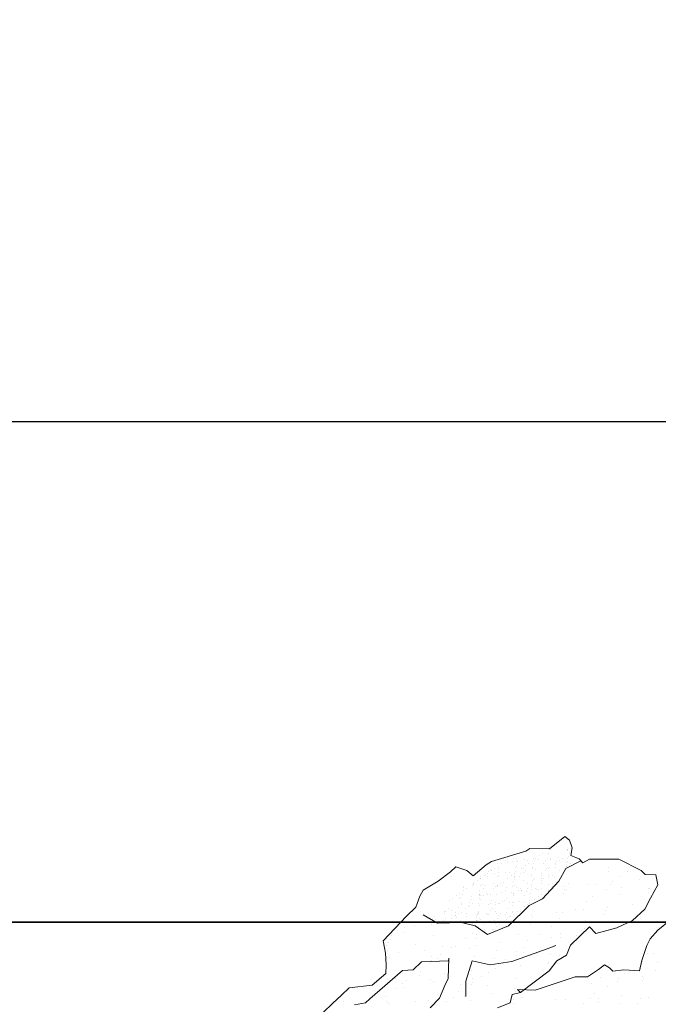
# Model space of a CAD drawing. Units: inches. Extents: x 1986 to 21484, y -1816 to 2016.
# Tile 76 of 85: x 3645 to 3661, y 1899 to 1924. Entities that reach past the tile are written whole.
import ezdxf

# ---------------------------------------------------------------- set-up
doc = ezdxf.new("R2010")
doc.units = ezdxf.units.IN
for name, color, linetype, lineweight in [('A-ANNO-DIMS', 2, 'Continuous', 18), ('C-PROP', 7, 'Continuous', 35), ('L-PLNT', 84, 'Continuous', 13)]:
    doc.layers.add(name, color=color, linetype=linetype, lineweight=lineweight)
doc.styles.get("Standard").update_dxf_attribs({"font": 'arial.ttf'})
doc.dimstyles.new('ISO-25', dxfattribs={"dimtxt": 8, "dimasz": 2.5, "dimexe": 1.25, "dimexo": 0.625, "dimtad": 1, "dimdec": 1, "dimlunit": 3, "dimtxsty": 'Standard', "dimcen": 2.5, "dimadec": 0, "dimazin": 0, "dimtfac": 1, "dimtdec": 1, "dimtmove": 0, "dimatfit": 3, "dimfxl": 1, "dimarcsym": 0})

# ---------------------------------------------------------------- blocks, each defined once
blk = doc.blocks.new('*D33')
at = {"layer": 'A-ANNO-DIMS', "color": 0, "lineweight": -2, "transparency": 16777216}
for p, q in [((3538.907, 1901.377), (3538.907, 1914.655)), ((3898.907, 1901.377), (3898.907, 1914.655)), ((3541.407, 1913.405), (3896.407, 1913.405))]:
    blk.add_line(p, q, dxfattribs=at)
at = {"layer": 'A-ANNO-DIMS', "color": 0, "transparency": 16777216}
for points in [[(3541.407, 1913.821), (3541.407, 1912.988), (3538.907, 1913.405)], [(3896.407, 1913.821), (3896.407, 1912.988), (3898.907, 1913.405)]]:
    blk.add_solid(points, dxfattribs=at)
at = {"layer": 'Defpoints', "color": 0, "transparency": 16777216}
for p in [(3898.907, 1913.405), (3538.907, 1900.752), (3898.907, 1900.752)]:
    blk.add_point(p, dxfattribs=at)
at = {"layer": 'A-ANNO-DIMS', "color": 0, "transparency": 16777216, "insert": (3718.907, 1918.117), "char_height": 8, "attachment_point": 5}
blk.add_mtext("30'", dxfattribs=at)
blk = doc.blocks.new('PLANT-SHRUB')
for p, q in [((2159.692, 1873.568), (2159.692, 1873.568)), ((2160.01, 1873.488), (2160.01, 1873.488)), ((2159.852, 1873.457), (2159.852, 1873.457)), ((2158.917, 1873.074), (2158.917, 1873.074)), ((2159.085, 1873.181), (2159.085, 1873.181)), ((2159.431, 1873.071), (2159.431, 1873.071)), ((2159.446, 1873.132), (2159.446, 1873.132)), ((2159.504, 1873.138), (2159.504, 1873.138)), ((2160.161, 1873.071), (2160.161, 1873.071)), ((2160.33, 1873.179), (2160.33, 1873.179)), ((2159.17, 1872.773), (2158.818, 1872.576)), ((2158.845, 1872.837), (2158.845, 1872.837)), ((2158.939, 1872.731), (2158.939, 1872.731)), ((2159.398, 1872.918), (2159.17, 1872.773)), ((2159.17, 1872.794), (2159.17, 1872.794)), ((2159.667, 1872.628), (2159.398, 1872.918)), ((2160.706, 1872.787), (2160.706, 1872.787)), ((2158.352, 1872.483), (2157.948, 1872.514)), ((2158.642, 1872.514), (2158.352, 1872.483)), ((2158.818, 1872.576), (2158.642, 1872.514)), ((2159.033, 1872.706), (2159.033, 1872.706)), ((2159.895, 1872.463), (2159.667, 1872.628)), ((2159.713, 1872.723), (2159.713, 1872.723)), ((2159.921, 1872.695), (2159.921, 1872.695)), ((2159.985, 1872.718), (2159.985, 1872.718)), ((2160.245, 1872.652), (2160.245, 1872.652)), ((2160.614, 1872.565), (2160.614, 1872.565)), ((2160.632, 1872.72), (2160.632, 1872.72)), ((2160.788, 1872.581), (2160.788, 1872.581)), ((2160.996, 1872.554), (2160.996, 1872.554)), ((2159.895, 1872.349), (2159.895, 1872.463)), ((2159.936, 1872.204), (2159.895, 1872.349)), ((2160.234, 1872.355), (2160.234, 1872.355)), ((2160.5, 1872.323), (2160.5, 1872.323)), ((2160.123, 1872.183), (2159.936, 1872.204)), ((2160.454, 1872.131), (2160.123, 1872.183)), ((2160.682, 1871.914), (2160.454, 1872.131)), ((2161.252, 1872.176), (2161.252, 1872.176)), ((2161.436, 1872.005), (2161.436, 1872.005)), ((2157.565, 1871.655), (2157.937, 1871.769)), ((2157.937, 1871.769), (2158.227, 1871.873)), ((2158.227, 1871.873), (2158.652, 1871.873)), ((2158.227, 1871.873), (2158.227, 1871.873)), ((2158.652, 1871.873), (2159.066, 1871.738)), ((2158.801, 1871.808), (2158.801, 1871.808)), ((2159.066, 1871.738), (2159.553, 1871.479)), ((2160.682, 1871.914), (2160.682, 1871.914)), ((2161.656, 1871.469), (2160.682, 1871.914)), ((2157.43, 1871.428), (2157.565, 1871.655)), ((2157.792, 1871.569), (2157.792, 1871.569)), ((2157.802, 1871.568), (2157.802, 1871.568)), ((2157.866, 1871.637), (2157.866, 1871.637)), ((2158.373, 1871.586), (2158.373, 1871.586)), ((2159.046, 1871.566), (2159.046, 1871.566)), ((2161.536, 1871.561), (2161.536, 1871.561)), ((2157.43, 1871.428), (2157.43, 1871.428)), ((2157.627, 1871.241), (2157.43, 1871.428)), ((2157.627, 1871.096), (2157.627, 1871.241)), ((2159.067, 1871.286), (2159.067, 1871.286)), ((2159.553, 1871.479), (2159.553, 1871.241)), ((2159.553, 1871.241), (2160.226, 1871.252)), ((2160.226, 1871.252), (2160.465, 1871.366)), ((2160.465, 1871.366), (2160.744, 1871.303)), ((2160.617, 1871.254), (2160.617, 1871.254)), ((2160.744, 1871.303), (2161.065, 1871.355)), ((2161.065, 1871.355), (2161.966, 1871.262)), ((2161.966, 1871.148), (2161.656, 1871.469)), ((2161.704, 1871.426), (2161.704, 1871.426)), ((2161.966, 1871.262), (2162.152, 1871.148)), ((2161.966, 1871.262), (2161.966, 1871.148)), ((2162.029, 1871.383), (2162.029, 1871.383)), ((2162.152, 1871.148), (2162.339, 1871.269)), ((2162.216, 1871.268), (2162.216, 1871.268)), ((2162.29, 1871.335), (2162.29, 1871.335)), ((2162.339, 1871.269), (2162.651, 1871.144)), ((2157.844, 1870.507), (2157.627, 1871.096)), ((2157.809, 1871.23), (2157.809, 1871.23)), ((2158.271, 1871.072), (2158.271, 1871.072)), ((2158.44, 1871.179), (2158.44, 1871.179)), ((2158.888, 1871.191), (2158.888, 1871.191)), ((2158.994, 1871.219), (2158.994, 1871.219)), ((2159.516, 1871.07), (2159.516, 1871.07)), ((2159.684, 1871.177), (2159.684, 1871.177)), ((2159.935, 1871.178), (2159.935, 1871.178)), ((2160.498, 1871.004), (2160.717, 1870.911)), ((2160.76, 1871.068), (2160.76, 1871.068)), ((2160.929, 1871.175), (2160.929, 1871.175)), ((2160.957, 1871.183), (2160.957, 1871.183)), ((2162.005, 1871.065), (2162.005, 1871.065)), ((2162.036, 1871.144), (2162.036, 1871.144)), ((2162.174, 1871.173), (2162.174, 1871.173)), ((2157.9, 1870.892), (2157.9, 1870.892)), ((2158.108, 1870.864), (2158.108, 1870.864)), ((2158.348, 1870.816), (2158.348, 1870.816)), ((2158.433, 1870.821), (2158.433, 1870.821)), ((2158.596, 1870.854), (2158.596, 1870.854)), ((2158.976, 1870.75), (2158.976, 1870.75)), ((2159.37, 1870.821), (2159.37, 1870.821)), ((2160.195, 1870.868), (2160.195, 1870.868)), ((2160.269, 1870.935), (2160.269, 1870.935)), ((2160.45, 1870.782), (2160.45, 1870.782)), ((2160.717, 1870.911), (2161.59, 1870.537)), ((2161.496, 1870.769), (2161.496, 1870.769)), ((2161.818, 1870.903), (2161.818, 1870.903)), ((2162.518, 1870.774), (2162.518, 1870.774)), ((2157.844, 1870.507), (2157.844, 1870.507)), ((2158.384, 1869.997), (2157.844, 1870.507)), ((2158.248, 1870.535), (2158.248, 1870.535)), ((2158.724, 1870.565), (2158.724, 1870.565)), ((2159.184, 1870.723), (2159.184, 1870.723)), ((2159.508, 1870.68), (2159.508, 1870.68)), ((2159.797, 1870.503), (2159.797, 1870.503)), ((2159.968, 1870.563), (2159.968, 1870.563)), ((2160.051, 1870.608), (2160.051, 1870.608)), ((2160.259, 1870.581), (2160.259, 1870.581)), ((2160.584, 1870.538), (2160.584, 1870.538)), ((2161.213, 1870.561), (2161.213, 1870.561)), ((2161.397, 1870.517), (2161.397, 1870.517)), ((2161.47, 1870.584), (2161.47, 1870.584)), ((2161.59, 1870.537), (2162.042, 1870.225)), ((2162.458, 1870.558), (2162.458, 1870.558)), ((2163.02, 1870.552), (2163.02, 1870.552)), ((2158.175, 1870.468), (2158.175, 1870.468)), ((2158.863, 1870.421), (2158.863, 1870.421)), ((2159.909, 1870.408), (2159.909, 1870.408)), ((2160.932, 1870.413), (2160.932, 1870.413)), ((2161.127, 1870.467), (2161.127, 1870.467)), ((2161.335, 1870.439), (2161.335, 1870.439)), ((2161.66, 1870.396), (2161.66, 1870.396)), ((2162.011, 1870.374), (2162.011, 1870.374)), ((2162.203, 1870.325), (2162.203, 1870.325)), ((2162.411, 1870.298), (2162.411, 1870.298)), ((2162.736, 1870.255), (2162.736, 1870.255)), ((2162.775, 1870.1), (2163.041, 1870.381)), ((2163.057, 1870.36), (2163.057, 1870.36)), ((2158.323, 1870.046), (2158.323, 1870.046)), ((2158.384, 1869.997), (2158.384, 1869.997)), ((2158.57, 1869.945), (2158.384, 1869.997)), ((2159.193, 1870.069), (2159.193, 1870.069)), ((2159.345, 1870.051), (2159.345, 1870.051)), ((2159.362, 1870.176), (2159.362, 1870.176)), ((2159.376, 1870.117), (2159.376, 1870.117)), ((2159.45, 1870.185), (2159.45, 1870.185)), ((2160.425, 1870.012), (2160.425, 1870.012)), ((2160.438, 1870.067), (2160.438, 1870.067)), ((2160.606, 1870.174), (2160.606, 1870.174)), ((2160.999, 1870.152), (2160.999, 1870.152)), ((2161.471, 1869.999), (2161.471, 1869.999)), ((2161.682, 1870.064), (2161.682, 1870.064)), ((2161.851, 1870.172), (2161.851, 1870.172)), ((2162.042, 1870.225), (2162.308, 1869.835)), ((2162.308, 1869.835), (2162.775, 1870.1)), ((2162.493, 1870.004), (2162.493, 1870.004)), ((2162.598, 1870.166), (2162.598, 1870.166)), ((2162.672, 1870.234), (2162.672, 1870.234)), ((2162.927, 1870.062), (2162.927, 1870.062)), ((2163.095, 1870.17), (2163.095, 1870.17)), ((2163.279, 1870.183), (2163.279, 1870.183)), ((2163.487, 1870.156), (2163.487, 1870.156)), ((2158.57, 1869.81), (2158.57, 1869.945)), ((2158.57, 1869.878), (2158.986, 1869.757)), ((2158.663, 1869.603), (2158.57, 1869.81)), ((2158.607, 1869.764), (2158.607, 1869.764)), ((2158.978, 1869.753), (2158.978, 1869.753)), ((2158.986, 1869.757), (2159.329, 1869.866)), ((2159.329, 1869.866), (2159.937, 1869.913)), ((2159.451, 1869.859), (2159.451, 1869.859)), ((2159.534, 1869.849), (2159.534, 1869.849)), ((2159.579, 1869.872), (2159.579, 1869.872)), ((2159.588, 1869.751), (2159.588, 1869.751)), ((2159.664, 1869.831), (2159.664, 1869.831)), ((2159.672, 1869.868), (2159.672, 1869.868)), ((2159.747, 1869.897), (2159.747, 1869.897)), ((2159.881, 1869.803), (2159.881, 1869.803)), ((2159.937, 1869.913), (2160.296, 1869.804)), ((2159.965, 1869.792), (2159.965, 1869.792)), ((2159.988, 1869.874), (2159.988, 1869.874)), ((2160.095, 1869.775), (2160.095, 1869.775)), ((2160.228, 1869.757), (2160.228, 1869.757)), ((2160.258, 1869.784), (2160.258, 1869.784)), ((2160.296, 1869.804), (2161.029, 1869.82)), ((2160.296, 1869.804), (2160.296, 1869.804)), ((2160.312, 1869.746), (2160.312, 1869.746)), ((2160.578, 1869.766), (2160.578, 1869.766)), ((2160.651, 1869.834), (2160.651, 1869.834)), ((2160.877, 1869.771), (2160.877, 1869.771)), ((2161.029, 1869.82), (2161.575, 1869.617)), ((2162.2, 1869.802), (2162.2, 1869.802)), ((2163.243, 1869.82), (2163.056, 1869.742)), ((2163.555, 1869.96), (2163.243, 1869.82)), ((2163.898, 1869.976), (2163.555, 1869.96)), ((2163.573, 1869.965), (2163.573, 1869.965)), ((2163.8, 1869.815), (2163.8, 1869.815)), ((2158.508, 1869.49), (2158.663, 1869.603)), ((2158.615, 1869.513), (2158.615, 1869.513)), ((2158.656, 1869.55), (2158.656, 1869.55)), ((2158.663, 1869.603), (2158.663, 1869.603)), ((2158.719, 1869.585), (2158.719, 1869.585)), ((2158.78, 1869.591), (2158.78, 1869.591)), ((2158.815, 1869.736), (2158.815, 1869.736)), ((2158.838, 1869.651), (2158.838, 1869.651)), ((2158.858, 1869.667), (2158.858, 1869.667)), ((2158.873, 1869.522), (2158.873, 1869.522)), ((2158.939, 1869.737), (2158.939, 1869.737)), ((2158.944, 1869.727), (2158.944, 1869.727)), ((2158.957, 1869.511), (2158.957, 1869.511)), ((2159.113, 1869.512), (2159.113, 1869.512)), ((2159.14, 1869.693), (2159.14, 1869.693)), ((2159.15, 1869.569), (2159.15, 1869.569)), ((2159.353, 1869.729), (2159.353, 1869.729)), ((2159.355, 1869.667), (2159.355, 1869.667)), ((2159.42, 1869.597), (2159.42, 1869.597)), ((2159.449, 1869.624), (2159.449, 1869.624)), ((2159.569, 1869.564), (2159.569, 1869.564)), ((2159.611, 1869.511), (2159.611, 1869.511)), ((2159.646, 1869.562), (2159.646, 1869.562)), ((2159.683, 1869.622), (2159.683, 1869.622)), ((2159.785, 1869.714), (2159.785, 1869.714)), ((2159.853, 1869.666), (2159.853, 1869.666)), ((2159.884, 1869.638), (2159.884, 1869.638)), ((2159.891, 1869.595), (2159.891, 1869.595)), ((2159.978, 1869.566), (2159.978, 1869.566)), ((2160.069, 1869.611), (2160.069, 1869.611)), ((2160.108, 1869.51), (2160.108, 1869.51)), ((2160.203, 1869.708), (2160.203, 1869.708)), ((2160.216, 1869.552), (2160.216, 1869.552)), ((2160.351, 1869.665), (2160.351, 1869.665)), ((2160.395, 1869.735), (2160.395, 1869.735)), ((2160.41, 1869.55), (2160.41, 1869.55)), ((2160.525, 1869.718), (2160.525, 1869.718)), ((2160.606, 1869.509), (2160.606, 1869.509)), ((2160.612, 1869.71), (2160.612, 1869.71)), ((2160.709, 1869.616), (2160.709, 1869.616)), ((2160.738, 1869.643), (2160.738, 1869.643)), ((2160.742, 1869.69), (2160.742, 1869.69)), ((2160.825, 1869.679), (2160.825, 1869.679)), ((2160.828, 1869.545), (2160.828, 1869.545)), ((2160.849, 1869.664), (2160.849, 1869.664)), ((2160.89, 1869.56), (2160.89, 1869.56)), ((2160.907, 1869.642), (2160.907, 1869.642)), ((2160.955, 1869.661), (2160.955, 1869.661)), ((2161.044, 1869.695), (2161.044, 1869.695)), ((2161.104, 1869.508), (2161.104, 1869.508)), ((2161.172, 1869.633), (2161.172, 1869.633)), ((2161.219, 1869.503), (2161.219, 1869.503)), ((2161.237, 1869.547), (2161.237, 1869.547)), ((2161.256, 1869.622), (2161.256, 1869.622)), ((2161.347, 1869.663), (2161.347, 1869.663)), ((2161.358, 1869.63), (2161.358, 1869.63)), ((2161.386, 1869.605), (2161.386, 1869.605)), ((2161.575, 1869.617), (2161.652, 1869.243)), ((2161.986, 1869.604), (2161.986, 1869.604)), ((2162.135, 1869.558), (2162.135, 1869.558)), ((2163.056, 1869.742), (2162.697, 1869.383)), ((2163.032, 1869.59), (2163.032, 1869.59)), ((2163.056, 1869.742), (2163.056, 1869.742)), ((2163.379, 1869.555), (2163.379, 1869.555)), ((2164.055, 1869.595), (2164.055, 1869.595)), ((2158.425, 1869.303), (2158.508, 1869.49)), ((2158.446, 1869.148), (2158.425, 1869.303)), ((2158.548, 1869.47), (2158.548, 1869.47)), ((2158.612, 1869.437), (2158.612, 1869.437)), ((2158.631, 1869.434), (2158.631, 1869.434)), ((2158.641, 1869.464), (2158.641, 1869.464)), ((2158.934, 1869.419), (2158.934, 1869.419)), ((2159.045, 1869.469), (2159.045, 1869.469)), ((2159.087, 1869.494), (2159.087, 1869.494)), ((2159.092, 1869.296), (2159.092, 1869.296)), ((2159.122, 1869.323), (2159.122, 1869.323)), ((2159.14, 1869.261), (2159.14, 1869.261)), ((2159.226, 1869.266), (2159.226, 1869.266)), ((2159.261, 1869.451), (2159.261, 1869.451)), ((2159.304, 1869.465), (2159.304, 1869.465)), ((2159.32, 1869.281), (2159.32, 1869.281)), ((2159.343, 1869.421), (2159.343, 1869.421)), ((2159.387, 1869.454), (2159.387, 1869.454)), ((2159.517, 1869.437), (2159.517, 1869.437)), ((2159.543, 1869.468), (2159.543, 1869.468)), ((2159.559, 1869.256), (2159.559, 1869.256)), ((2159.724, 1869.265), (2159.724, 1869.265)), ((2159.734, 1869.408), (2159.734, 1869.408)), ((2159.741, 1869.31), (2159.741, 1869.31)), ((2159.775, 1869.406), (2159.775, 1869.406)), ((2159.817, 1869.397), (2159.817, 1869.397)), ((2159.9, 1869.456), (2159.9, 1869.456)), ((2159.93, 1869.483), (2159.93, 1869.483)), ((2159.947, 1869.38), (2159.947, 1869.38)), ((2159.968, 1869.258), (2159.968, 1869.258)), ((2160.041, 1869.467), (2160.041, 1869.467)), ((2160.164, 1869.352), (2160.164, 1869.352)), ((2160.18, 1869.402), (2160.18, 1869.402)), ((2160.193, 1869.4), (2160.193, 1869.4)), ((2160.222, 1869.264), (2160.222, 1869.264)), ((2160.248, 1869.341), (2160.248, 1869.341)), ((2160.377, 1869.324), (2160.377, 1869.324)), ((2160.381, 1869.316), (2160.381, 1869.316)), ((2160.41, 1869.343), (2160.41, 1869.343)), ((2160.539, 1869.466), (2160.539, 1869.466)), ((2160.55, 1869.47), (2160.55, 1869.47)), ((2160.595, 1869.295), (2160.595, 1869.295)), ((2160.602, 1869.402), (2160.602, 1869.402)), ((2160.678, 1869.284), (2160.678, 1869.284)), ((2160.72, 1869.264), (2160.72, 1869.264)), ((2160.759, 1869.48), (2160.759, 1869.48)), ((2160.808, 1869.267), (2160.808, 1869.267)), ((2160.967, 1869.453), (2160.967, 1869.453)), ((2161.03, 1869.33), (2161.03, 1869.33)), ((2161.034, 1869.387), (2161.034, 1869.387)), ((2161.037, 1869.465), (2161.037, 1869.465)), ((2161.189, 1869.476), (2161.189, 1869.476)), ((2161.218, 1869.263), (2161.218, 1869.263)), ((2161.292, 1869.41), (2161.292, 1869.41)), ((2161.453, 1869.381), (2161.453, 1869.381)), ((2161.535, 1869.464), (2161.535, 1869.464)), ((2161.779, 1869.416), (2161.779, 1869.416)), ((2161.835, 1869.339), (2161.835, 1869.339)), ((2161.853, 1869.483), (2161.853, 1869.483)), ((2162.043, 1869.311), (2162.043, 1869.311)), ((2162.367, 1869.269), (2162.367, 1869.269)), ((2162.697, 1869.383), (2162.744, 1869.43)), ((2162.744, 1869.43), (2163.259, 1868.978)), ((2163.402, 1869.451), (2163.402, 1869.451)), ((2158.943, 1869.107), (2158.446, 1869.148)), ((2158.933, 1869.151), (2158.933, 1869.151)), ((2159.305, 1868.765), (2158.943, 1869.107)), ((2158.984, 1869.112), (2158.984, 1869.112)), ((2159.039, 1869.176), (2159.039, 1869.176)), ((2159.156, 1869.07), (2159.156, 1869.07)), ((2159.239, 1869.059), (2159.239, 1869.059)), ((2159.333, 1869.113), (2159.333, 1869.113)), ((2159.369, 1869.042), (2159.369, 1869.042)), ((2159.414, 1869.068), (2159.414, 1869.068)), ((2159.414, 1869.01), (2159.414, 1869.01)), ((2159.482, 1869.111), (2159.482, 1869.111)), ((2159.573, 1869.156), (2159.573, 1869.156)), ((2159.587, 1869.014), (2159.587, 1869.014)), ((2159.602, 1869.183), (2159.602, 1869.183)), ((2159.67, 1869.003), (2159.67, 1869.003)), ((2159.758, 1869.016), (2159.758, 1869.016)), ((2159.765, 1869.098), (2159.765, 1869.098)), ((2159.832, 1869.083), (2159.832, 1869.083)), ((2159.912, 1869.067), (2159.912, 1869.067)), ((2159.979, 1869.11), (2159.979, 1869.11)), ((2160.053, 1869.016), (2160.053, 1869.016)), ((2160.083, 1869.043), (2160.083, 1869.043)), ((2160.115, 1869.066), (2160.115, 1869.066)), ((2160.183, 1869.092), (2160.183, 1869.092)), ((2160.222, 1869.17), (2160.222, 1869.17)), ((2160.283, 1869.173), (2160.283, 1869.173)), ((2160.4, 1869.242), (2160.4, 1869.242)), ((2160.4, 1869.242), (2160.4, 1869.242)), ((2160.41, 1869.066), (2160.41, 1869.066)), ((2160.477, 1869.109), (2160.477, 1869.109)), ((2160.592, 1869.094), (2160.592, 1869.094)), ((2160.702, 1869.03), (2160.702, 1869.03)), ((2160.818, 1869.237), (2160.818, 1869.237)), ((2160.862, 1869.176), (2160.862, 1869.176)), ((2160.891, 1869.203), (2160.891, 1869.203)), ((2160.908, 1869.065), (2160.908, 1869.065)), ((2160.975, 1869.108), (2160.975, 1869.108)), ((2161.024, 1869.079), (2161.024, 1869.079)), ((2161.025, 1869.238), (2161.025, 1869.238)), ((2161.108, 1869.227), (2161.108, 1869.227)), ((2161.227, 1869.239), (2161.227, 1869.239)), ((2161.238, 1869.21), (2161.238, 1869.21)), ((2161.342, 1869.035), (2161.342, 1869.035)), ((2161.359, 1869.064), (2161.359, 1869.064)), ((2161.372, 1869.062), (2161.372, 1869.062)), ((2161.381, 1869.051), (2161.381, 1869.051)), ((2161.406, 1869.064), (2161.406, 1869.064)), ((2161.443, 1869.073), (2161.443, 1869.073)), ((2161.446, 1869.229), (2161.446, 1869.229)), ((2161.455, 1869.182), (2161.455, 1869.182)), ((2161.473, 1869.107), (2161.473, 1869.107)), ((2161.511, 1869.19), (2161.511, 1869.19)), ((2161.528, 1869.171), (2161.528, 1869.171)), ((2161.539, 1869.171), (2161.539, 1869.171)), ((2161.652, 1869.243), (2161.84, 1868.947)), ((2161.659, 1869.223), (2161.659, 1869.223)), ((2161.668, 1869.154), (2161.668, 1869.154)), ((2162.468, 1869.234), (2162.468, 1869.234)), ((2162.604, 1869.061), (2162.604, 1869.061)), ((2162.773, 1869.169), (2162.773, 1869.169)), ((2162.91, 1869.197), (2162.91, 1869.197)), ((2162.98, 1869.065), (2162.98, 1869.065)), ((2163.054, 1869.132), (2163.054, 1869.132)), ((2163.118, 1869.17), (2163.118, 1869.17)), ((2163.443, 1869.127), (2163.443, 1869.127)), ((2163.548, 1869.195), (2163.548, 1869.195)), ((2163.849, 1869.059), (2163.849, 1869.059)), ((2163.986, 1869.055), (2163.986, 1869.055)), ((2164.017, 1869.167), (2164.017, 1869.167)), ((2164.194, 1869.028), (2164.194, 1869.028)), ((2164.594, 1869.181), (2164.594, 1869.181)), ((2164.603, 1869.1), (2164.603, 1869.1)), ((2159.419, 1868.745), (2159.305, 1868.765)), ((2159.549, 1868.948), (2159.549, 1868.948)), ((2159.595, 1868.865), (2159.595, 1868.865)), ((2159.755, 1868.79), (2159.755, 1868.79)), ((2159.8, 1868.986), (2159.8, 1868.986)), ((2159.859, 1868.867), (2159.859, 1868.867)), ((2159.894, 1868.87), (2159.894, 1868.87)), ((2159.958, 1868.95), (2159.958, 1868.95)), ((2160.017, 1868.957), (2160.017, 1868.957)), ((2160.093, 1868.864), (2160.093, 1868.864)), ((2160.1, 1868.946), (2160.1, 1868.946)), ((2160.173, 1868.784), (2160.173, 1868.784)), ((2160.23, 1868.929), (2160.23, 1868.929)), ((2160.389, 1868.934), (2160.389, 1868.934)), ((2160.447, 1868.9), (2160.447, 1868.9)), ((2160.53, 1868.89), (2160.53, 1868.89)), ((2160.534, 1868.875), (2160.534, 1868.875)), ((2160.563, 1868.902), (2160.563, 1868.902)), ((2160.582, 1868.786), (2160.582, 1868.786)), ((2160.591, 1868.863), (2160.591, 1868.863)), ((2160.66, 1868.872), (2160.66, 1868.872)), ((2160.808, 1868.929), (2160.808, 1868.929)), ((2160.878, 1868.844), (2160.878, 1868.844)), ((2160.881, 1868.872), (2160.881, 1868.872)), ((2160.961, 1868.833), (2160.961, 1868.833)), ((2161.014, 1868.771), (2161.014, 1868.771)), ((2161.044, 1868.762), (2161.044, 1868.762)), ((2161.089, 1868.862), (2161.089, 1868.862)), ((2161.091, 1868.816), (2161.091, 1868.816)), ((2161.183, 1868.89), (2161.183, 1868.89)), ((2161.217, 1868.931), (2161.217, 1868.931)), ((2161.308, 1868.787), (2161.308, 1868.787)), ((2161.391, 1868.776), (2161.391, 1868.776)), ((2161.432, 1868.765), (2161.432, 1868.765)), ((2161.521, 1868.759), (2161.521, 1868.759)), ((2161.587, 1868.861), (2161.587, 1868.861)), ((2161.649, 1868.915), (2161.649, 1868.915)), ((2161.664, 1868.749), (2161.664, 1868.749)), ((2161.823, 1868.895), (2161.823, 1868.895)), ((2161.84, 1868.947), (2162.292, 1868.542)), ((2161.841, 1868.767), (2161.841, 1868.767)), ((2161.852, 1868.922), (2161.852, 1868.922)), ((2161.961, 1868.833), (2161.961, 1868.833)), ((2163.007, 1868.82), (2163.007, 1868.82)), ((2163.259, 1868.978), (2163.555, 1868.978)), ((2163.259, 1868.978), (2163.259, 1868.978)), ((2163.555, 1868.978), (2163.758, 1868.807)), ((2163.758, 1868.807), (2164.852, 1868.768)), ((2163.758, 1868.807), (2163.758, 1868.807)), ((2164.03, 1868.825), (2164.03, 1868.825)), ((2164.256, 1868.781), (2164.256, 1868.781)), ((2164.519, 1868.985), (2164.519, 1868.985)), ((2164.852, 1868.768), (2165.004, 1868.762)), ((2165.004, 1868.762), (2165.237, 1868.611)), ((2160.231, 1868.339), (2159.419, 1868.745)), ((2159.726, 1868.715), (2159.726, 1868.715)), ((2159.755, 1868.742), (2159.755, 1868.742)), ((2159.783, 1868.667), (2159.783, 1868.667)), ((2159.85, 1868.709), (2159.85, 1868.709)), ((2159.87, 1868.563), (2159.87, 1868.563)), ((2159.948, 1868.642), (2159.948, 1868.642)), ((2159.953, 1868.552), (2159.953, 1868.552)), ((2160.083, 1868.535), (2160.083, 1868.535)), ((2160.206, 1868.575), (2160.206, 1868.575)), ((2160.236, 1868.602), (2160.236, 1868.602)), ((2160.281, 1868.666), (2160.281, 1868.666)), ((2160.3, 1868.506), (2160.3, 1868.506)), ((2160.348, 1868.709), (2160.348, 1868.709)), ((2160.375, 1868.73), (2160.375, 1868.73)), ((2160.379, 1868.626), (2160.379, 1868.626)), ((2160.567, 1868.559), (2160.567, 1868.559)), ((2160.779, 1868.665), (2160.779, 1868.665)), ((2160.798, 1868.621), (2160.798, 1868.621)), ((2160.846, 1868.708), (2160.846, 1868.708)), ((2160.855, 1868.589), (2160.855, 1868.589)), ((2160.96, 1868.665), (2160.96, 1868.665)), ((2161.014, 1868.735), (2161.014, 1868.735)), ((2161.033, 1868.732), (2161.033, 1868.732)), ((2161.207, 1868.623), (2161.207, 1868.623)), ((2161.276, 1868.664), (2161.276, 1868.664)), ((2161.344, 1868.707), (2161.344, 1868.707)), ((2161.495, 1868.595), (2161.495, 1868.595)), ((2161.525, 1868.622), (2161.525, 1868.622)), ((2161.639, 1868.607), (2161.639, 1868.607)), ((2161.738, 1868.731), (2161.738, 1868.731)), ((2161.774, 1868.663), (2161.774, 1868.663)), ((2161.812, 1868.557), (2161.812, 1868.557)), ((2161.821, 1868.72), (2161.821, 1868.72)), ((2161.842, 1868.706), (2161.842, 1868.706)), ((2161.951, 1868.702), (2161.951, 1868.702)), ((2162.057, 1868.602), (2162.057, 1868.602)), ((2162.144, 1868.609), (2162.144, 1868.609)), ((2162.292, 1868.542), (2162.417, 1868.137)), ((2162.583, 1868.7), (2162.583, 1868.7)), ((2163.057, 1868.555), (2163.057, 1868.555)), ((2164.117, 1868.578), (2163.962, 1868.423)), ((2164.117, 1868.578), (2164.117, 1868.578)), ((2164.573, 1868.557), (2164.117, 1868.578)), ((2164.182, 1868.714), (2164.182, 1868.714)), ((2164.301, 1868.552), (2164.301, 1868.552)), ((2164.573, 1868.557), (2164.573, 1868.557)), ((2165.041, 1868.204), (2164.573, 1868.557)), ((2160.163, 1868.476), (2160.163, 1868.476)), ((2160.386, 1868.307), (2160.231, 1868.339)), ((2160.374, 1868.472), (2160.374, 1868.472)), ((2160.383, 1868.495), (2160.383, 1868.495)), ((2160.821, 1868.287), (2160.386, 1868.307)), ((2160.39, 1868.494), (2160.39, 1868.494)), ((2160.462, 1868.463), (2160.462, 1868.463)), ((2160.513, 1868.478), (2160.513, 1868.478)), ((2160.572, 1868.478), (2160.572, 1868.478)), ((2160.598, 1868.467), (2160.598, 1868.467)), ((2160.687, 1868.435), (2160.687, 1868.435)), ((2160.716, 1868.462), (2160.716, 1868.462)), ((2160.717, 1868.307), (2160.717, 1868.307)), ((2160.73, 1868.449), (2160.73, 1868.449)), ((2160.788, 1868.313), (2160.788, 1868.313)), ((2160.813, 1868.438), (2160.813, 1868.438)), ((2160.842, 1868.08), (2160.821, 1868.287)), ((2160.923, 1868.424), (2160.923, 1868.424)), ((2160.943, 1868.421), (2160.943, 1868.421)), ((2160.96, 1868.462), (2160.96, 1868.462)), ((2161.004, 1868.463), (2161.004, 1868.463)), ((2161.16, 1868.393), (2161.16, 1868.393)), ((2161.197, 1868.321), (2161.197, 1868.321)), ((2161.197, 1868.315), (2161.197, 1868.315)), ((2161.244, 1868.382), (2161.244, 1868.382)), ((2161.336, 1868.449), (2161.336, 1868.449)), ((2161.374, 1868.365), (2161.374, 1868.365)), ((2161.421, 1868.459), (2161.421, 1868.459)), ((2161.422, 1868.457), (2161.422, 1868.457)), ((2161.457, 1868.461), (2161.457, 1868.461)), ((2161.466, 1868.352), (2161.466, 1868.352)), ((2161.591, 1868.336), (2161.591, 1868.336)), ((2161.674, 1868.325), (2161.674, 1868.325)), ((2161.674, 1868.325), (2161.674, 1868.325)), ((2161.831, 1868.459), (2161.831, 1868.459)), ((2161.955, 1868.46), (2161.955, 1868.46)), ((2161.976, 1868.454), (2161.976, 1868.454)), ((2162.005, 1868.481), (2162.005, 1868.481)), ((2162.235, 1868.382), (2162.235, 1868.382)), ((2162.263, 1868.444), (2162.263, 1868.444)), ((2162.443, 1868.464), (2162.443, 1868.464)), ((2163.522, 1868.425), (2163.522, 1868.425)), ((2163.962, 1868.423), (2163.775, 1868.195)), ((2163.784, 1868.349), (2163.784, 1868.349)), ((2163.962, 1868.423), (2163.962, 1868.423)), ((2165.383, 1868.363), (2165.383, 1868.363)), ((2160.987, 1867.821), (2160.842, 1868.08)), ((2162.75, 1868.183), (2162.75, 1868.183)), ((2162.982, 1868.05), (2162.982, 1868.05)), ((2163.075, 1868.141), (2163.075, 1868.141)), ((2163.436, 1868.031), (2163.436, 1868.031)), ((2163.526, 1868.058), (2163.526, 1868.058)), ((2163.703, 1868.081), (2163.599, 1867.926)), ((2163.618, 1868.069), (2163.618, 1868.069)), ((2163.695, 1868.166), (2163.695, 1868.166)), ((2163.775, 1868.195), (2163.703, 1868.081)), ((2163.703, 1868.081), (2163.703, 1868.081)), ((2165.041, 1868.204), (2165.041, 1868.204)), ((2165.311, 1868.204), (2165.041, 1868.204)), ((2165.621, 1868.204), (2165.311, 1868.204)), ((2166.253, 1868.214), (2165.621, 1868.204)), ((2161.163, 1867.821), (2160.987, 1867.821)), ((2161.557, 1867.78), (2161.163, 1867.821)), ((2161.992, 1867.687), (2161.557, 1867.78)), ((2162.416, 1867.873), (2162.158, 1867.738)), ((2162.748, 1867.873), (2162.416, 1867.873)), ((2163.599, 1867.926), (2162.748, 1867.873)), ((2162.748, 1867.873), (2162.748, 1867.873)), ((2163.363, 1867.963), (2163.363, 1867.963)), ((2162.158, 1867.738), (2161.992, 1867.687))]:
    blk.add_line(p, q)

msp = doc.modelspace()

# ---------------------------------------------------------------- linework, layer by layer
at = {"layer": 'C-PROP'}
msp.add_lwpolyline([(3538.907, 1900.752), (3898.907, 1900.752), (3898.907, 1066.752), (3538.907, 1066.752)], close=True, dxfattribs=at)

# ---------------------------------------------------------------- block references
at = {"layer": 'L-PLNT', "rotation": 223.1883365522388}
msp.add_blockref('PLANT-SHRUB', (3953.27, 4742.965), dxfattribs=at)

# ---------------------------------------------------------------- dimensions: what is measured, and where the dimension line sits
at = {"layer": 'A-ANNO-DIMS'}
dim = msp.add_linear_dim(base=(3898.907, 1913.405), p1=(3538.907, 1900.752), p2=(3898.907, 1900.752), dimstyle='ISO-25', override={"dimclrd": 0, "dimclre": 0, "dimclrt": 0}, dxfattribs=at)
dim.commit()
dim.dimension.update_dxf_attribs({"geometry": '*D33', "text_midpoint": (3718.907, 1918.117)})

doc.saveas('drawing.dxf')
